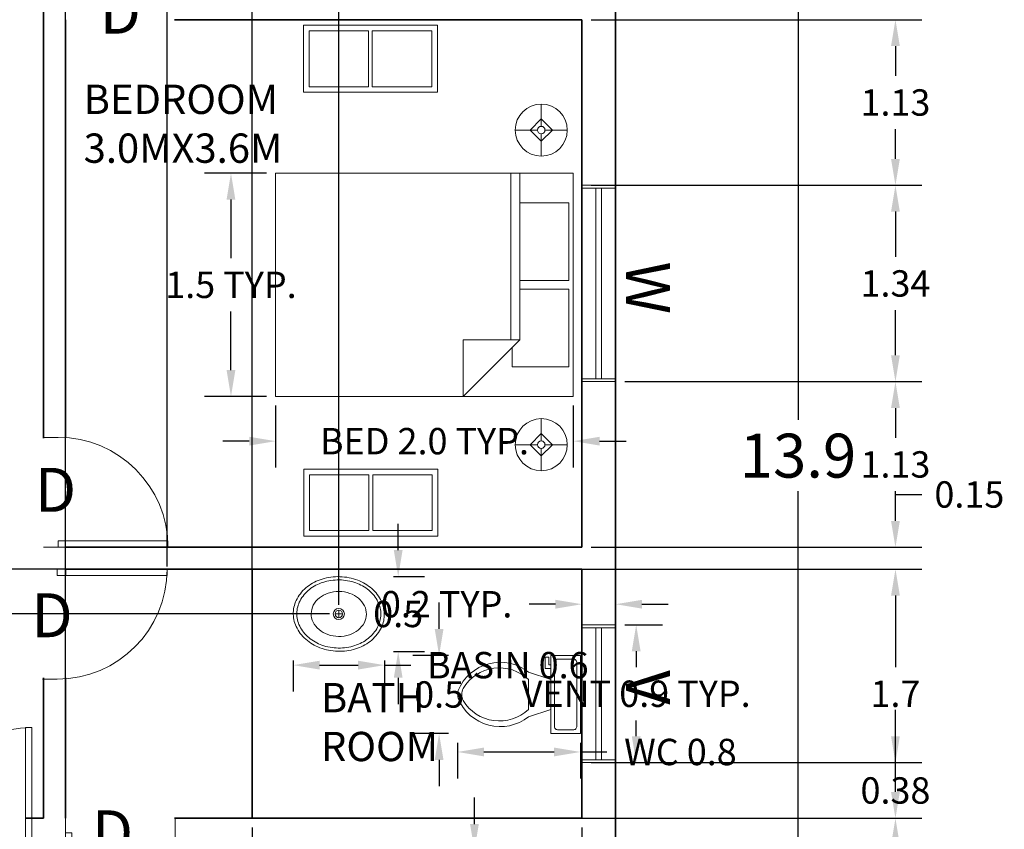
# Model space of a CAD drawing. Units: metres. Extents: x 40.9 to 56.1, y -1.4 to 24.2.
# Tile 5 of 7: x 48.4 to 55.2, y 13.1 to 18.6. Entities that reach past the tile are written whole.
import ezdxf

# ---------------------------------------------------------------- set-up
doc = ezdxf.new("R2010")
doc.units = ezdxf.units.M
doc.header["$MEASUREMENT"] = 0
for name, color, linetype, lineweight in [('A-ANNO-DIMS', 2, 'Continuous', 18), ('A-ANNO-TEXT', 7, 'Continuous', 18), ('A-AREA-IDEN', 7, 'Continuous', 18), ('A-DOOR', 3, 'Continuous', 18), ('A-FLOR-CASE', 9, 'Continuous', 18), ('A-FLOR-FIXT', 9, 'Continuous', 18), ('A-FURN', 8, 'Continuous', 18), ('A-GLAZ', 4, 'Continuous', 18), ('A-WALL', 7, 'Continuous', 35)]:
    doc.layers.add(name, color=color, linetype=linetype, lineweight=lineweight)
doc.styles.get("Standard").update_dxf_attribs({"font": 'arial.ttf'})
doc.dimstyles.get("Standard").update_dxf_attribs({"dimtxt": 0.18, "dimasz": 0.18, "dimexe": 0.18, "dimexo": 0.0625, "dimgap": 0.09, "dimtad": 0, "dimtih": 1, "dimtoh": 1, "dimdec": 1, "dimzin": 0, "dimdsep": 46, "dimtxsty": 'Standard', "dimcen": 0.09, "dimadec": 0, "dimazin": 0, "dimtfac": 1, "dimtdec": 1, "dimtofl": 0, "dimtmove": 0, "dimatfit": 3, "dimfxl": 1, "dimtolj": 1, "dimtzin": 0, "dimarcsym": 0})

# ---------------------------------------------------------------- blocks, each defined once
blk = doc.blocks.new('*U3')
for p, q in [((-750, 0), (-750, -100)), ((0, 0), (0, -100))]:
    blk.add_line(p, q)
blk.add_lwpolyline([(0, 0), (0, 750), (-43.75, 750), (-43.75, 0)], close=True)
blk.add_arc((0, 0), 750, 90, 180)
blk = doc.blocks.new('*U4')
for p, q in [((0, 0), (0, 100)), ((750, 0), (750, 100))]:
    blk.add_line(p, q)
blk.add_lwpolyline([(0, 0), (0, -750), (43.75, -750), (43.75, 0)], close=True)
blk.add_arc((0, 0), 750, 270, 0)
blk = doc.blocks.new('*U5')
for p, q in [((-750, 0), (-750, 100)), ((0, 0), (0, 100))]:
    blk.add_line(p, q)
blk.add_lwpolyline([(0, 0), (0, -750), (-43.75, -750), (-43.75, 0)], close=True)
blk.add_arc((0, 0), 750, 180, 270)
blk = doc.blocks.new('*U6')
for p, q in [((0, 0), (0, 100)), ((750, 0), (750, 100))]:
    blk.add_line(p, q)
blk.add_lwpolyline([(0, 0), (0, -750), (43.75, -750), (43.75, 0)], close=True)
blk.add_arc((0, 0), 750, 270, 0)
blk = doc.blocks.new('Bed - Queen')
for p, q in [((0, -80.00003), (0, 0)), ((0, 0), (59.99999, 0)), ((59.99999, 0), (59.99999, -80.00003)), ((7.99999, -1.2), (28.79998, -1.2)), ((7.99999, -14.4), (7.99999, -1.2)), ((28.79998, -1.2), (28.79998, -14.4)), ((31.19999, -1.2), (51.99999, -1.2)), ((31.19999, -14.4), (31.19999, -1.2)), ((51.99999, -1.2), (51.99999, -16.4)), ((0, -14.4), (44.8, -14.4)), ((59.99999, -29.6), (44.8, -14.4)), ((44.8, -14.4), (44.8, -29.6)), ((44.8, -16.8), (0, -16.8)), ((51.99999, -16.4), (46.79936, -16.4)), ((44.8, -29.6), (59.99999, -29.6)), ((59.99999, -80.00003), (0, -80.00003))]:
    blk.add_line(p, q)
blk = doc.blocks.new('Lamp - Table')
for p, q in [((0, 7), (0, 1)), ((0, 3), (-3, 0)), ((3, 0), (0, 3)), ((-1, 0), (-7, 0)), ((-3, 0), (0, -3)), ((0, -3), (3, 0)), ((1, 0), (7, 0)), ((0, -1), (0, -7))]:
    blk.add_line(p, q)
for radius in [7, 1]:
    blk.add_circle((0, 0), radius)
blk = doc.blocks.new('Toilet - top')
for p, q in [((9.5, -6), (9.5, -2)), ((-10, -8.5), (-8, -8.5)), ((-10, -9.5), (-10, -8.5)), ((-7, -9.5), (-10, -9.5)), ((-8, -8.5), (-8, -8)), ((-7, -8), (-7, -9.5)), ((-4, -8), (-6, -14)), ((4, -8), (6, -14)), ((4, -14), (-4, -14))]:
    blk.add_line(p, q)
blk.add_lwpolyline([(10.5, -8), (10.5, 0), (-10.5, 0), (-10.5, -8)], close=True)
for points in [[(-9.5, -2), (-9.5, -6)], [(8.5, -1), (-8.5, -1)], [(-8.5, -7), (8.5, -7)]]:
    blk.add_lwpolyline(points)
for centre, radius, start, end in [((-8.62, -1.88), 0.884, 81.8699, 188.1301), ((8.62, -1.88), 0.884, 351.8699, 98.1301), ((-8.62, -6.12), 0.884, 171.8699, 278.1301), ((8.62, -6.12), 0.884, 261.8699, 8.1301), ((3.52, -21.58), 12.17, 141.4691, 247.9714), ((4.2, -21.82), 11.33, 136.3677, 238.9468), ((-3.52, -21.58), 12.17, 292.0284, 38.5307), ((-4.2, -21.82), 11.33, 301.053, 43.6321), ((0, -27.88), 4, 245.7318, 294.2682), ((0, -29), 4, 254.8605, 285.1395)]:
    blk.add_arc(centre, radius, start, end)
blk = doc.blocks.new('Sink - Oval top')
for p, q in [((-1, 0), (1, 0)), ((0, 1), (0, -1))]:
    blk.add_line(p, q)
for points in [[(-12.23, 0.39, 0.117634), (-11.46, -3.36, 0.104469), (-8.88, -6.8, 0.090016), (-5.08, -9.07, 0.08192), (-0.32, -10.02, 0.08192), (4.49, -9.38, 0.090016), (8.42, -7.36, 0.104469), (11.22, -4.09, 0.117634), (12.23, -0.39, 0.117634), (11.46, 3.36, 0.104469), (8.88, 6.8, 0.090016), (5.08, 9.07, 0.08192), (0.32, 10.02, 0.08192), (-4.49, 9.38, 0.090016), (-8.42, 7.36, 0.104469), (-11.22, 4.09, 0.117634)], [(-11.29, 0.16, 0.118622), (-10.52, -3.25, 0.104678), (-8.07, -6.36, 0.089562), (-4.54, -8.37, 0.081185), (-0.13, -9.15, 0.081185), (4.3, -8.49, 0.089562), (7.89, -6.58, 0.104678), (10.42, -3.55, 0.118622), (11.29, -0.16, 0.118622), (10.52, 3.25, 0.104678), (8.07, 6.36, 0.089562), (4.54, 8.37, 0.081185), (0.13, 9.15, 0.081185), (-4.3, 8.49, 0.089562), (-7.89, 6.58, 0.104678), (-10.42, 3.55, 0.118622)], [(-7.42, 0.08, 0.118283), (-6.91, -2.17, 0.104607), (-5.29, -4.21, 0.089718), (-2.97, -5.53, 0.081436), (-0.07, -6.04, 0.081436), (2.84, -5.59, 0.089718), (5.2, -4.33, 0.104607), (6.86, -2.32, 0.118283), (7.42, -0.08, 0.118283), (6.91, 2.17, 0.104607), (5.29, 4.21, 0.089718), (2.97, 5.53, 0.081436), (0.07, 6.04, 0.081436), (-2.84, 5.59, 0.089718), (-5.2, 4.33, 0.104607), (-6.86, 2.32, 0.118283)]]:
    blk.add_lwpolyline(points, format="xyb", close=True)
for radius in [1.5, 1]:
    blk.add_circle((0, 0), radius)
blk = doc.blocks.new('Wall Cabinet - 18 x 36 in front')
for p, q in [((17.5, -1.5), (17.5, -16.5)), ((18.5, -16.5), (18.5, -1.5))]:
    blk.add_line(p, q)
blk.add_lwpolyline([(0, -18), (0, 0), (36, 0), (36, -18)], close=True)
for points in [[(17.5, -16.5), (1.5, -16.5), (1.5, -1.5), (17.5, -1.5)], [(18.5, -1.5), (34.5, -1.5), (34.5, -16.5), (18.5, -16.5)]]:
    blk.add_lwpolyline(points)
blk = doc.blocks.new('*D46')
at = {"layer": 'A-ANNO-DIMS', "color": 0, "lineweight": -2, "transparency": 16777216}
for p, q in [((52.5777, 22.5873), (53.9408, 22.5873)), ((53.7608, 22.2873), (53.7608, 15.8755)), ((53.7608, 8.9773), (53.7608, 15.389)), ((52.5777, 8.6773), (53.9408, 8.6773))]:
    blk.add_line(p, q, dxfattribs=at)
at = {"layer": 'A-ANNO-DIMS', "color": 0, "transparency": 16777216}
for points in [[(53.7108, 22.2873), (53.8108, 22.2873), (53.7608, 22.5873)], [(53.7108, 8.9773), (53.8108, 8.9773), (53.7608, 8.6773)]]:
    blk.add_solid(points, dxfattribs=at)
at = {"layer": 'Defpoints', "color": 0, "transparency": 16777216}
for p in [(52.5152, 22.5873), (52.5152, 8.6773), (53.7608, 8.6773)]:
    blk.add_point(p, dxfattribs=at)
at = {"layer": 'A-ANNO-DIMS', "color": 0, "transparency": 16777216, "insert": (53.7608, 15.6323), "char_height": 0.3, "attachment_point": 5}
blk.add_mtext('\\A1;13.9', dxfattribs=at)
blk = doc.blocks.new('VENT-900-PLAN')
for p, q in [((0.0002, 0.0003), (0.0002, 0.2303)), ((0.0202, 0.0003), (0.0202, 0.2303)), ((0.9202, 0.0003), (0.9202, 0.2303)), ((0.9402, 0.0003), (0.9402, 0.2303)), ((0.0202, 0.1353), (0.9202, 0.1353)), ((0.0202, 0.0953), (0.9202, 0.0953))]:
    blk.add_line(p, q)
blk = doc.blocks.new('*D75')
at = {"layer": 'A-ANNO-DIMS', "color": 0, "lineweight": -2, "transparency": 16777216}
for p, q in [((52.5777, 14.4773), (52.8362, 14.4773)), ((52.6562, 14.2973), (52.6562, 14.1892)), ((52.6562, 13.7173), (52.6562, 13.8254)), ((52.5777, 13.5373), (52.8362, 13.5373))]:
    blk.add_line(p, q, dxfattribs=at)
at = {"layer": 'A-ANNO-DIMS', "color": 0, "transparency": 16777216}
for points in [[(52.6262, 14.2973), (52.6862, 14.2973), (52.6562, 14.4773)], [(52.6262, 13.7173), (52.6862, 13.7173), (52.6562, 13.5373)]]:
    blk.add_solid(points, dxfattribs=at)
at = {"layer": 'Defpoints', "color": 0, "transparency": 16777216}
for p in [(52.5152, 14.4773), (52.6562, 14.4773), (52.5152, 13.5373)]:
    blk.add_point(p, dxfattribs=at)
at = {"layer": 'A-ANNO-DIMS', "color": 0, "transparency": 16777216, "insert": (52.6562, 14.0073), "char_height": 0.18, "attachment_point": 5}
blk.add_mtext('\\A1;VENT 0.9 TYP.', dxfattribs=at)
blk = doc.blocks.new('*D76')
at = {"layer": 'A-ANNO-DIMS', "color": 0, "lineweight": -2, "transparency": 16777216}
for p, q in [((52.2852, 14.5398), (52.2852, 14.7983)), ((52.5152, 14.5398), (52.5152, 14.7983)), ((52.1052, 14.6183), (51.9252, 14.6183)), ((52.6952, 14.6183), (52.8752, 14.6183))]:
    blk.add_line(p, q, dxfattribs=at)
at = {"layer": 'A-ANNO-DIMS', "color": 0, "transparency": 16777216}
for points in [[(52.1052, 14.6483), (52.1052, 14.5883), (52.2852, 14.6183)], [(52.6952, 14.6483), (52.6952, 14.5883), (52.5152, 14.6183)]]:
    blk.add_solid(points, dxfattribs=at)
at = {"layer": 'Defpoints', "color": 0, "transparency": 16777216}
for p in [(52.2852, 14.6183), (52.2852, 14.4773), (52.5152, 14.4773)]:
    blk.add_point(p, dxfattribs=at)
at = {"layer": 'A-ANNO-DIMS', "color": 0, "transparency": 16777216, "insert": (51.3622, 14.6183), "char_height": 0.18, "attachment_point": 5}
blk.add_mtext('\\A1;0.2 TYP.', dxfattribs=at)
blk = doc.blocks.new('*D79')
at = {"layer": 'A-ANNO-DIMS', "color": 0, "lineweight": -2, "transparency": 16777216}
for p, q in [((50.1947, 15.9733), (50.1947, 15.551)), ((52.2267, 15.9733), (52.2267, 15.551)), ((50.0147, 15.731), (49.8347, 15.731)), ((52.4067, 15.731), (52.5867, 15.731))]:
    blk.add_line(p, q, dxfattribs=at)
at = {"layer": 'A-ANNO-DIMS', "color": 0, "transparency": 16777216}
for points in [[(50.0147, 15.761), (50.0147, 15.701), (50.1947, 15.731)], [(52.4067, 15.761), (52.4067, 15.701), (52.2267, 15.731)]]:
    blk.add_solid(points, dxfattribs=at)
at = {"layer": 'Defpoints', "color": 0, "transparency": 16777216}
for p in [(50.1947, 16.0358), (52.2267, 16.0358), (52.2267, 15.731)]:
    blk.add_point(p, dxfattribs=at)
at = {"layer": 'A-ANNO-DIMS', "color": 0, "transparency": 16777216, "insert": (51.2107, 15.731), "char_height": 0.18, "attachment_point": 5}
blk.add_mtext('\\A1;BED 2.0 TYP.', dxfattribs=at)
blk = doc.blocks.new('*D80')
at = {"layer": 'A-ANNO-DIMS', "color": 0, "lineweight": -2, "transparency": 16777216}
for p, q in [((50.1322, 17.5598), (49.7099, 17.5598)), ((49.8899, 17.3798), (49.8899, 16.9798)), ((49.8899, 16.2158), (49.8899, 16.6159)), ((50.1322, 16.0358), (49.7099, 16.0358))]:
    blk.add_line(p, q, dxfattribs=at)
at = {"layer": 'A-ANNO-DIMS', "color": 0, "transparency": 16777216}
for points in [[(49.8599, 17.3798), (49.9199, 17.3798), (49.8899, 17.5598)], [(49.8599, 16.2158), (49.9199, 16.2158), (49.8899, 16.0358)]]:
    blk.add_solid(points, dxfattribs=at)
at = {"layer": 'Defpoints', "color": 0, "transparency": 16777216}
for p in [(50.1947, 17.5598), (49.8899, 16.0358), (50.1947, 16.0358)]:
    blk.add_point(p, dxfattribs=at)
at = {"layer": 'A-ANNO-DIMS', "color": 0, "transparency": 16777216, "insert": (49.8899, 16.7978), "char_height": 0.18, "attachment_point": 5}
blk.add_mtext('\\A1;1.5 TYP.', dxfattribs=at)
blk = doc.blocks.new('*D86')
at = {"layer": 'A-ANNO-DIMS', "color": 0, "lineweight": -2, "transparency": 16777216}
for p, q in [((51.5519, 13.1183), (51.5519, 13.2983)), ((51.4772, 12.9383), (51.7319, 12.9383)), ((51.4772, 12.4811), (51.7319, 12.4811)), ((51.5519, 12.3011), (51.5519, 12.1211))]:
    blk.add_line(p, q, dxfattribs=at)
at = {"layer": 'A-ANNO-DIMS', "color": 0, "transparency": 16777216}
for points in [[(51.5219, 13.1183), (51.5819, 13.1183), (51.5519, 12.9383)], [(51.5219, 12.3011), (51.5819, 12.3011), (51.5519, 12.4811)]]:
    blk.add_solid(points, dxfattribs=at)
at = {"layer": 'Defpoints', "color": 0, "transparency": 16777216}
for p in [(51.4147, 12.9383), (51.5519, 12.9383), (51.4147, 12.4811)]:
    blk.add_point(p, dxfattribs=at)
at = {"layer": 'A-ANNO-DIMS', "color": 0, "transparency": 16777216, "insert": (51.5519, 12.7097), "char_height": 0.18, "attachment_point": 5}
blk.add_mtext('\\A1;0.5 TYP.', dxfattribs=at)
blk = doc.blocks.new('*D91')
at = {"layer": 'A-ANNO-DIMS', "color": 0, "lineweight": -2, "transparency": 16777216}
for p, q in [((51.4367, 13.6733), (51.4367, 13.4299)), ((52.2761, 13.6733), (52.2761, 13.4299)), ((51.6167, 13.6099), (52.0961, 13.6099)), ((52.2761, 13.6099), (52.4561, 13.6099))]:
    blk.add_line(p, q, dxfattribs=at)
at = {"layer": 'A-ANNO-DIMS', "color": 0, "transparency": 16777216}
for points in [[(51.6167, 13.6399), (51.6167, 13.5799), (51.4367, 13.6099)], [(52.0961, 13.6399), (52.0961, 13.5799), (52.2761, 13.6099)]]:
    blk.add_solid(points, dxfattribs=at)
at = {"layer": 'Defpoints', "color": 0, "transparency": 16777216}
for p in [(51.4367, 13.7358), (52.2761, 13.7358), (52.2761, 13.6099)]:
    blk.add_point(p, dxfattribs=at)
at = {"layer": 'A-ANNO-DIMS', "color": 0, "transparency": 16777216, "insert": (52.9582, 13.6099), "char_height": 0.18, "attachment_point": 5}
blk.add_mtext('\\A1;WC 0.8', dxfattribs=at)
blk = doc.blocks.new('*D92')
at = {"layer": 'A-ANNO-DIMS', "color": 0, "lineweight": -2, "transparency": 16777216}
for p, q in [((51.3108, 14.4492), (51.3108, 14.6292)), ((51.3742, 14.2692), (51.1308, 14.2692)), ((51.3742, 13.7358), (51.1308, 13.7358)), ((51.3108, 13.5558), (51.3108, 13.3758))]:
    blk.add_line(p, q, dxfattribs=at)
at = {"layer": 'A-ANNO-DIMS', "color": 0, "transparency": 16777216}
for points in [[(51.2808, 14.4492), (51.3408, 14.4492), (51.3108, 14.2692)], [(51.2808, 13.5558), (51.3408, 13.5558), (51.3108, 13.7358)]]:
    blk.add_solid(points, dxfattribs=at)
at = {"layer": 'Defpoints', "color": 0, "transparency": 16777216}
for p in [(51.4367, 14.2692), (51.3108, 13.7358), (51.4367, 13.7358)]:
    blk.add_point(p, dxfattribs=at)
at = {"layer": 'A-ANNO-DIMS', "color": 0, "transparency": 16777216, "insert": (51.3108, 14.0025), "char_height": 0.18, "attachment_point": 5}
blk.add_mtext('\\A1;0.5', dxfattribs=at)
blk = doc.blocks.new('*D95')
at = {"layer": 'A-ANNO-DIMS', "color": 0, "lineweight": -2, "transparency": 16777216}
for p, q in [((50.3144, 14.2336), (50.3144, 14.0225)), ((50.4944, 14.2025), (50.7579, 14.2025)), ((50.9379, 14.2336), (50.9379, 14.0225)), ((50.9379, 14.2025), (51.1179, 14.2025))]:
    blk.add_line(p, q, dxfattribs=at)
at = {"layer": 'A-ANNO-DIMS', "color": 0, "transparency": 16777216}
for points in [[(50.4944, 14.2325), (50.4944, 14.1725), (50.3144, 14.2025)], [(50.7579, 14.2325), (50.7579, 14.1725), (50.9379, 14.2025)]]:
    blk.add_solid(points, dxfattribs=at)
at = {"layer": 'Defpoints', "color": 0, "transparency": 16777216}
for p in [(50.3144, 14.2961), (50.9379, 14.2961), (50.9379, 14.2025)]:
    blk.add_point(p, dxfattribs=at)
at = {"layer": 'A-ANNO-DIMS', "color": 0, "transparency": 16777216, "insert": (51.78, 14.2025), "char_height": 0.18, "attachment_point": 5}
blk.add_mtext('\\A1;BASIN 0.6', dxfattribs=at)
blk = doc.blocks.new('*D96')
at = {"layer": 'A-ANNO-DIMS', "color": 0, "lineweight": -2, "transparency": 16777216}
for p, q in [((51.0315, 14.9875), (51.0315, 15.1675)), ((51.0004, 14.8075), (51.2115, 14.8075)), ((51.0004, 14.2961), (51.2115, 14.2961)), ((51.0315, 14.1161), (51.0315, 13.9361))]:
    blk.add_line(p, q, dxfattribs=at)
at = {"layer": 'A-ANNO-DIMS', "color": 0, "transparency": 16777216}
for points in [[(51.0015, 14.9875), (51.0615, 14.9875), (51.0315, 14.8075)], [(51.0015, 14.1161), (51.0615, 14.1161), (51.0315, 14.2961)]]:
    blk.add_solid(points, dxfattribs=at)
at = {"layer": 'Defpoints', "color": 0, "transparency": 16777216}
for p in [(50.9379, 14.8075), (51.0315, 14.8075), (50.9379, 14.2961)]:
    blk.add_point(p, dxfattribs=at)
at = {"layer": 'A-ANNO-DIMS', "color": 0, "transparency": 16777216, "insert": (51.0315, 14.5518), "char_height": 0.18, "attachment_point": 5}
blk.add_mtext('\\A1;0.5', dxfattribs=at)
blk = doc.blocks.new('*D134')
at = {"layer": 'A-ANNO-DIMS', "color": 0, "lineweight": -2, "transparency": 16777216}
for p, q in [((50.034, 13.0948), (50.034, 6.6791)), ((52.2852, 13.0948), (52.2852, 6.6791)), ((50.214, 6.8591), (50.8336, 6.8591)), ((52.1052, 6.8591), (51.4856, 6.8591))]:
    blk.add_line(p, q, dxfattribs=at)
at = {"layer": 'A-ANNO-DIMS', "color": 0, "transparency": 16777216}
for points in [[(50.214, 6.8891), (50.214, 6.8291), (50.034, 6.8591)], [(52.1052, 6.8891), (52.1052, 6.8291), (52.2852, 6.8591)]]:
    blk.add_solid(points, dxfattribs=at)
at = {"layer": 'Defpoints', "color": 0, "transparency": 16777216}
for p in [(50.034, 13.1573), (52.2852, 13.1573), (52.2852, 6.8591)]:
    blk.add_point(p, dxfattribs=at)
at = {"layer": 'A-ANNO-DIMS', "color": 0, "transparency": 16777216, "insert": (51.1596, 6.8591), "char_height": 0.18, "attachment_point": 5}
blk.add_mtext('\\A1;2.25', dxfattribs=at)
blk = doc.blocks.new('*D135')
at = {"layer": 'A-ANNO-DIMS', "color": 0, "lineweight": -2, "transparency": 16777216}
for p, q in [((50.0965, 14.8573), (54.6058, 14.8573)), ((54.4258, 14.6773), (54.4258, 14.1876)), ((54.4258, 13.3373), (54.4258, 13.8269)), ((50.0965, 13.1573), (54.6058, 13.1573))]:
    blk.add_line(p, q, dxfattribs=at)
at = {"layer": 'A-ANNO-DIMS', "color": 0, "transparency": 16777216}
for points in [[(54.3958, 14.6773), (54.4558, 14.6773), (54.4258, 14.8573)], [(54.3958, 13.3373), (54.4558, 13.3373), (54.4258, 13.1573)]]:
    blk.add_solid(points, dxfattribs=at)
at = {"layer": 'Defpoints', "color": 0, "transparency": 16777216}
for p in [(50.034, 14.8573), (54.4258, 14.8573), (50.034, 13.1573)]:
    blk.add_point(p, dxfattribs=at)
at = {"layer": 'A-ANNO-DIMS', "color": 0, "transparency": 16777216, "insert": (54.4258, 14.0073), "char_height": 0.18, "attachment_point": 5}
blk.add_mtext('\\A1;1.7', dxfattribs=at)
blk = doc.blocks.new('*D136')
at = {"layer": 'A-ANNO-DIMS', "color": 0, "lineweight": -2, "transparency": 16777216}
for p, q in [((48.7602, 14.8764), (48.7602, 24.2418)), ((49.4546, 14.8764), (49.4546, 24.2418)), ((48.5802, 24.0618), (48.4002, 24.0618)), ((49.6346, 24.0618), (49.8146, 24.0618))]:
    blk.add_line(p, q, dxfattribs=at)
at = {"layer": 'A-ANNO-DIMS', "color": 0, "transparency": 16777216}
for points in [[(48.5802, 24.0918), (48.5802, 24.0318), (48.7602, 24.0618)], [(49.6346, 24.0918), (49.6346, 24.0318), (49.4546, 24.0618)]]:
    blk.add_solid(points, dxfattribs=at)
at = {"layer": 'Defpoints', "color": 0, "transparency": 16777216}
for p in [(49.4546, 24.0618), (48.7602, 14.8139), (49.4546, 14.8139)]:
    blk.add_point(p, dxfattribs=at)
at = {"layer": 'A-ANNO-DIMS', "color": 0, "transparency": 16777216, "insert": (49.1074, 24.0618), "char_height": 0.18, "attachment_point": 5}
blk.add_mtext('\\A1;0.69', dxfattribs=at)
blk = doc.blocks.new('*D140')
at = {"layer": 'A-ANNO-DIMS', "color": 0, "lineweight": -2, "transparency": 16777216}
for p, q in [((52.5777, 16.1373), (54.6058, 16.1373)), ((54.4258, 15.9573), (54.4258, 15.7542)), ((54.4258, 15.1873), (54.4258, 15.3903)), ((52.3477, 15.0073), (54.6058, 15.0073))]:
    blk.add_line(p, q, dxfattribs=at)
at = {"layer": 'A-ANNO-DIMS', "color": 0, "transparency": 16777216}
for points in [[(54.3958, 15.9573), (54.4558, 15.9573), (54.4258, 16.1373)], [(54.3958, 15.1873), (54.4558, 15.1873), (54.4258, 15.0073)]]:
    blk.add_solid(points, dxfattribs=at)
at = {"layer": 'Defpoints', "color": 0, "transparency": 16777216}
for p in [(52.5152, 16.1373), (54.4258, 16.1373), (52.2852, 15.0073)]:
    blk.add_point(p, dxfattribs=at)
at = {"layer": 'A-ANNO-DIMS', "color": 0, "transparency": 16777216, "insert": (54.4258, 15.5723), "char_height": 0.18, "attachment_point": 5}
blk.add_mtext('\\A1;1.13', dxfattribs=at)
blk = doc.blocks.new('*D141')
at = {"layer": 'A-ANNO-DIMS', "color": 0, "lineweight": -2, "transparency": 16777216}
for p, q in [((52.5777, 17.4773), (54.6058, 17.4773)), ((54.4258, 17.2973), (54.4258, 16.9892)), ((54.4258, 16.3173), (54.4258, 16.6253)), ((52.5777, 16.1373), (54.6058, 16.1373))]:
    blk.add_line(p, q, dxfattribs=at)
at = {"layer": 'A-ANNO-DIMS', "color": 0, "transparency": 16777216}
for points in [[(54.3958, 17.2973), (54.4558, 17.2973), (54.4258, 17.4773)], [(54.3958, 16.3173), (54.4558, 16.3173), (54.4258, 16.1373)]]:
    blk.add_solid(points, dxfattribs=at)
at = {"layer": 'Defpoints', "color": 0, "transparency": 16777216}
for p in [(52.5152, 17.4773), (54.4258, 17.4773), (52.5152, 16.1373)]:
    blk.add_point(p, dxfattribs=at)
at = {"layer": 'A-ANNO-DIMS', "color": 0, "transparency": 16777216, "insert": (54.4258, 16.8073), "char_height": 0.18, "attachment_point": 5}
blk.add_mtext('\\A1;1.34', dxfattribs=at)
blk = doc.blocks.new('*D150')
at = {"layer": 'A-ANNO-DIMS', "color": 0, "lineweight": -2, "transparency": 16777216}
for p, q in [((50.034, 14.9198), (50.034, 24.2418)), ((50.6262, 14.6143), (50.6262, 24.2418)), ((50.214, 24.0618), (50.4462, 24.0618)), ((50.6262, 24.0618), (50.8062, 24.0618))]:
    blk.add_line(p, q, dxfattribs=at)
at = {"layer": 'A-ANNO-DIMS', "color": 0, "transparency": 16777216}
for points in [[(50.214, 24.0918), (50.214, 24.0318), (50.034, 24.0618)], [(50.4462, 24.0918), (50.4462, 24.0318), (50.6262, 24.0618)]]:
    blk.add_solid(points, dxfattribs=at)
at = {"layer": 'Defpoints', "color": 0, "transparency": 16777216}
for p in [(50.6262, 24.0618), (50.034, 14.8573), (50.6262, 14.5518)]:
    blk.add_point(p, dxfattribs=at)
at = {"layer": 'A-ANNO-DIMS', "color": 0, "transparency": 16777216, "insert": (51.1301, 24.0618), "char_height": 0.18, "attachment_point": 5}
blk.add_mtext('\\A1;0.59', dxfattribs=at)
blk = doc.blocks.new('*D151')
at = {"layer": 'A-ANNO-DIMS', "color": 0, "lineweight": -2, "transparency": 16777216}
for p, q in [((43.3221, 15.0373), (43.3221, 15.2173)), ((49.9715, 14.8573), (43.1421, 14.8573)), ((50.5637, 14.5518), (43.1421, 14.5518)), ((43.3221, 14.3718), (43.3221, 14.1918)), ((43.3221, 14.1918), (43.1421, 14.1918))]:
    blk.add_line(p, q, dxfattribs=at)
at = {"layer": 'A-ANNO-DIMS', "color": 0, "transparency": 16777216}
for points in [[(43.2921, 15.0373), (43.3521, 15.0373), (43.3221, 14.8573)], [(43.2921, 14.3718), (43.3521, 14.3718), (43.3221, 14.5518)]]:
    blk.add_solid(points, dxfattribs=at)
at = {"layer": 'Defpoints', "color": 0, "transparency": 16777216}
for p in [(50.034, 14.8573), (43.3221, 14.5518), (50.6262, 14.5518)]:
    blk.add_point(p, dxfattribs=at)
at = {"layer": 'A-ANNO-DIMS', "color": 0, "transparency": 16777216, "insert": (42.8357, 14.1918), "char_height": 0.18, "attachment_point": 5}
blk.add_mtext('\\A1;0.31', dxfattribs=at)
blk = doc.blocks.new('*D152')
at = {"layer": 'A-ANNO-DIMS', "color": 0, "lineweight": -2, "transparency": 16777216}
for p, q in [((54.42584, 13.717253), (54.42584, 13.897253)), ((52.347703, 13.537253), (54.60584, 13.537253)), ((52.347703, 13.157253), (54.60584, 13.157253)), ((54.42584, 12.977253), (54.42584, 12.797253))]:
    blk.add_line(p, q, dxfattribs=at)
at = {"layer": 'A-ANNO-DIMS', "color": 0, "transparency": 16777216}
for points in [[(54.39584, 13.717253), (54.45584, 13.717253), (54.42584, 13.537253)], [(54.39584, 12.977253), (54.45584, 12.977253), (54.42584, 13.157253)]]:
    blk.add_solid(points, dxfattribs=at)
at = {"layer": 'Defpoints', "color": 0, "transparency": 16777216}
for p in [(52.285203, 13.537253), (54.42584, 13.537253), (52.285203, 13.157253)]:
    blk.add_point(p, dxfattribs=at)
at = {"layer": 'A-ANNO-DIMS', "color": 0, "transparency": 16777216, "insert": (54.42584, 13.347253), "char_height": 0.18, "attachment_point": 5}
blk.add_mtext('\\A1;0.38', dxfattribs=at)
blk = doc.blocks.new('*D153')
at = {"layer": 'A-ANNO-DIMS', "color": 0, "lineweight": -2, "transparency": 16777216}
for p, q in [((54.4258, 15.1873), (54.4258, 15.3673)), ((54.4258, 15.3673), (54.6058, 15.3673)), ((52.3477, 15.0073), (54.6058, 15.0073)), ((52.3477, 14.8573), (54.6058, 14.8573)), ((54.4258, 14.6773), (54.4258, 14.4973))]:
    blk.add_line(p, q, dxfattribs=at)
at = {"layer": 'A-ANNO-DIMS', "color": 0, "transparency": 16777216}
for points in [[(54.3958, 15.1873), (54.4558, 15.1873), (54.4258, 15.0073)], [(54.3958, 14.6773), (54.4558, 14.6773), (54.4258, 14.8573)]]:
    blk.add_solid(points, dxfattribs=at)
at = {"layer": 'Defpoints', "color": 0, "transparency": 16777216}
for p in [(52.2852, 15.0073), (54.4258, 15.0073), (52.2852, 14.8573)]:
    blk.add_point(p, dxfattribs=at)
at = {"layer": 'A-ANNO-DIMS', "color": 0, "transparency": 16777216, "insert": (54.9303, 15.3673), "char_height": 0.18, "attachment_point": 5}
blk.add_mtext('\\A1;0.15', dxfattribs=at)
blk = doc.blocks.new('*D154')
at = {"layer": 'A-ANNO-DIMS', "color": 0, "lineweight": -2, "transparency": 16777216}
for p, q in [((48.7602, 13.2198), (48.7602, 24.2418)), ((50.034, 13.2198), (50.034, 24.2418)), ((48.9402, 24.0618), (49.0818, 24.0618)), ((49.854, 24.0618), (49.7124, 24.0618))]:
    blk.add_line(p, q, dxfattribs=at)
at = {"layer": 'A-ANNO-DIMS', "color": 0, "transparency": 16777216}
for points in [[(48.9402, 24.0918), (48.9402, 24.0318), (48.7602, 24.0618)], [(49.854, 24.0918), (49.854, 24.0318), (50.034, 24.0618)]]:
    blk.add_solid(points, dxfattribs=at)
at = {"layer": 'Defpoints', "color": 0, "transparency": 16777216}
for p in [(50.034, 24.0618), (48.7602, 13.1573), (50.034, 13.1573)]:
    blk.add_point(p, dxfattribs=at)
at = {"layer": 'A-ANNO-DIMS', "color": 0, "transparency": 16777216, "insert": (49.3971, 24.0618), "char_height": 0.18, "attachment_point": 5}
blk.add_mtext('\\A1;1.27', dxfattribs=at)
blk = doc.blocks.new('*D159')
at = {"layer": 'A-ANNO-DIMS', "color": 0, "lineweight": -2, "transparency": 16777216}
for p, q in [((52.3477, 18.6073), (54.6058, 18.6073)), ((54.4258, 18.4273), (54.4258, 18.2242)), ((54.4258, 17.6573), (54.4258, 17.8603)), ((52.3477, 17.4773), (54.6058, 17.4773))]:
    blk.add_line(p, q, dxfattribs=at)
at = {"layer": 'A-ANNO-DIMS', "color": 0, "transparency": 16777216}
for points in [[(54.3958, 18.4273), (54.4558, 18.4273), (54.4258, 18.6073)], [(54.3958, 17.6573), (54.4558, 17.6573), (54.4258, 17.4773)]]:
    blk.add_solid(points, dxfattribs=at)
at = {"layer": 'Defpoints', "color": 0, "transparency": 16777216}
for p in [(52.2852, 18.6073), (54.4258, 18.6073), (52.2852, 17.4773)]:
    blk.add_point(p, dxfattribs=at)
at = {"layer": 'A-ANNO-DIMS', "color": 0, "transparency": 16777216, "insert": (54.4258, 18.0423), "char_height": 0.18, "attachment_point": 5}
blk.add_mtext('\\A1;1.13', dxfattribs=at)

msp = doc.modelspace()

# ---------------------------------------------------------------- linework, layer by layer
at = {"layer": 'A-GLAZ'}
for p, q in [((52.2852, 17.4773), (52.5152, 17.4773)), ((52.2852, 17.4573), (52.5152, 17.4573)), ((52.3802, 17.4573), (52.3802, 16.1573)), ((52.4202, 17.4573), (52.4202, 16.1573)), ((52.2852, 16.1573), (52.5152, 16.1573)), ((52.2852, 16.1373), (52.5152, 16.1373))]:
    msp.add_line(p, q, dxfattribs=at)
at = {"layer": 'A-WALL'}
for p, q in [((48.6102, 19.7073), (48.6102, 15.7504)), ((52.5152, 18.7573), (52.5152, 13.1573)), ((48.7602, 18.6073), (48.7602, 15.7554)), ((52.2852, 18.6073), (49.5035, 18.6073)), ((52.2852, 18.6073), (52.2852, 15.0073)), ((52.2852, 15.0073), (48.7602, 15.0073)), ((52.2852, 14.8573), (48.7602, 14.8573)), ((48.7602, 14.8573), (48.7602, 14.8139)), ((50.034, 14.8573), (50.034, 13.1573)), ((52.2852, 14.8573), (52.2852, 13.1573)), ((48.6102, 14.1157), (48.6102, 13.1573)), ((48.7602, 14.1157), (48.7602, 13.1573)), ((48.4865, 13.1573), (48.6102, 13.1573)), ((49.5035, 13.1573), (52.2852, 13.1573)), ((52.5152, 8.6773), (52.5152, 13.1573))]:
    msp.add_line(p, q, dxfattribs=at)

# ---------------------------------------------------------------- block references
at = {"layer": 'A-DOOR', "xscale": 0.001, "yscale": 0.001, "zscale": 0.001, "rotation": 90}
for name, p in [('*U6', (48.7102, 15.0071)), ('*U5', (48.7046, 14.8577))]:
    msp.add_blockref(name, p, dxfattribs=at)
at = {"layer": 'A-DOOR', "xscale": 0.001, "yscale": 0.001, "zscale": 0.001}
for name, p in [('*U3', (48.5302, 13.0273)), ('*U4', (48.7602, 13.0573))]:
    msp.add_blockref(name, p, dxfattribs=at)
at = {"layer": 'A-FLOR-CASE', "xscale": 0.0254, "yscale": 0.0254, "zscale": 0.0254}
for p in [(50.3846, 18.569), (50.3876, 15.5398)]:
    msp.add_blockref('Wall Cabinet - 18 x 36 in front', p, dxfattribs=at)
at = {"layer": 'A-FLOR-FIXT', "xscale": 0.0254, "yscale": 0.0254, "zscale": 0.0254}
msp.add_blockref('Sink - Oval top', (50.6262, 14.5518), dxfattribs=at)
at = {"layer": 'A-FLOR-FIXT', "xscale": 0.0254, "yscale": 0.0254, "zscale": 0.0254, "rotation": 270}
msp.add_blockref('Toilet - top', (52.2761, 14.0025), dxfattribs=at)
at = {"layer": 'A-FURN', "xscale": 0.0254, "yscale": 0.0254, "zscale": 0.0254}
for p in [(52.0082, 17.8539), (52.0082, 15.7069)]:
    msp.add_blockref('Lamp - Table', p, dxfattribs=at)
at = {"layer": 'A-FURN', "xscale": 0.0254, "yscale": 0.0254, "zscale": 0.0254, "rotation": 270}
msp.add_blockref('Bed - Queen', (52.2267, 17.5598), dxfattribs=at)
at = {"layer": 'A-GLAZ', "rotation": 90.0000000000022}
msp.add_blockref('VENT-900-PLAN', (52.5155, 13.5371), dxfattribs=at)

# ---------------------------------------------------------------- texts
at = {"layer": 'A-ANNO-TEXT'}
for p in [(48.994, 18.5117), (48.5518, 15.2488), (48.528, 14.3929), (48.9405, 12.9118)]:
    msp.add_text('D ', height=0.3, dxfattribs=at).set_placement(p)
for s, p in [('W', (52.5874, 16.9571)), ('V', (52.5874, 14.1683))]:
    msp.add_text(s, height=0.3, rotation=270, dxfattribs=at).set_placement(p)
at = {"layer": 'A-AREA-IDEN', "char_height": 0.2, "attachment_point": 1}
for s, insert in [('BEDROOM\\P3.0MX3.6M', (48.8846, 18.164)), ('BATH\\PROOM', (50.5047, 14.0807))]:
    msp.add_mtext_dynamic_manual_height_columns(s, width=2.030673, gutter_width=1, heights=[0], dxfattribs=dict(at, insert=insert))

# ---------------------------------------------------------------- dimensions: what is measured, and where the dimension line sits
at = {"layer": 'A-ANNO-DIMS'}
for base, p1, p2, picture, middle in [((49.4546, 24.0618), (48.7602, 14.8139), (49.4546, 14.8139), '*D136', (49.1074, 24.0618)), ((50.034, 24.0618), (48.7602, 13.1573), (50.034, 13.1573), '*D154', (49.3971, 24.0618)), ((50.6262, 24.0618), (50.034, 14.8573), (50.6262, 14.5518), '*D150', (51.1301, 24.0618)), ((52.2852, 6.8591), (50.034, 13.1573), (52.2852, 13.1573), '*D134', (51.1596, 6.8591))]:
    dim = msp.add_linear_dim(base=base, p1=p1, p2=p2, dimstyle='Standard', override={"dimdec": 2, "dimlfac": 1, "dimrnd": 0, "dimzin": 0, "dimdsep": 46, "dimlunit": 2}, dxfattribs=at)
    dim.commit()
    dim.dimension.update_dxf_attribs({"geometry": picture, "text_midpoint": middle})
for base, p1, p2, angle, override, picture, middle in [((53.7608, 8.6773), (52.5152, 22.5873), (52.5152, 8.6773), 90, {"dimtxt": 0.3, "dimasz": 0.3, "dimclrd": 0, "dimclre": 0, "dimclrt": 0}, '*D46', (53.7608, 15.6323)), ((54.4258, 18.6073), (52.2852, 17.4773), (52.2852, 18.6073), 90, {"dimdec": 2, "dimlfac": 1, "dimrnd": 0, "dimzin": 0, "dimdsep": 46, "dimlunit": 2}, '*D159', (54.4258, 18.0423)), ((54.4258, 17.4773), (52.5152, 16.1373), (52.5152, 17.4773), 90, {"dimdec": 2, "dimlfac": 1, "dimrnd": 0, "dimzin": 0, "dimdsep": 46, "dimlunit": 2}, '*D141', (54.4258, 16.8073)), ((54.4258, 16.1373), (52.2852, 15.0073), (52.5152, 16.1373), 90, {"dimdec": 2, "dimlfac": 1, "dimrnd": 0, "dimzin": 0, "dimdsep": 46, "dimlunit": 2}, '*D140', (54.4258, 15.5723)), ((54.4258, 15.0073), (52.2852, 14.8573), (52.2852, 15.0073), 90, {"dimdec": 2, "dimlfac": 1, "dimrnd": 0, "dimzin": 0, "dimdsep": 46, "dimlunit": 2}, '*D153', (54.9303, 15.3673)), ((43.3221, 14.5518), (50.034, 14.8573), (50.6262, 14.5518), 90, {"dimdec": 2, "dimlfac": 1, "dimrnd": 0, "dimzin": 0, "dimdsep": 46, "dimlunit": 2}, '*D151', (42.8357, 14.1918)), ((51.0315, 14.8075), (50.9379, 14.2961), (50.9379, 14.8075), 90, {"dimdec": 1, "dimlfac": 1, "dimrnd": 0, "dimzin": 0, "dimdsep": 46, "dimlunit": 2}, '*D96', (51.0315, 14.5518)), ((54.4258, 14.8573), (50.034, 13.1573), (50.034, 14.8573), 90, {"dimdec": 1, "dimlfac": 1, "dimrnd": 0, "dimzin": 0, "dimdsep": 46, "dimlunit": 2}, '*D135', (54.4258, 14.0073)), ((51.3108, 13.7358), (51.4367, 14.2692), (51.4367, 13.7358), 270, {"dimdec": 1, "dimlfac": 1, "dimrnd": 0, "dimzin": 0, "dimdsep": 46, "dimlunit": 2}, '*D92', (51.3108, 14.0025)), ((54.4258, 13.5373), (52.2852, 13.1573), (52.2852, 13.5373), 90, {"dimdec": 2, "dimlfac": 1, "dimrnd": 0, "dimzin": 0, "dimdsep": 46, "dimlunit": 2}, '*D152', (54.4258, 13.3473))]:
    dim = msp.add_linear_dim(base=base, p1=p1, p2=p2, angle=angle, dimstyle='Standard', override=override, dxfattribs=at)
    dim.commit()
    dim.dimension.update_dxf_attribs({"geometry": picture, "text_midpoint": middle})
for base, p1, p2, angle, text, picture, middle in [((49.8899, 16.0358), (50.1947, 17.5598), (50.1947, 16.0358), 270, '<> TYP.', '*D80', (49.8899, 16.7978)), ((52.2852, 14.6183), (52.5152, 14.4773), (52.2852, 14.4773), 180, '<> TYP.', '*D76', (51.3622, 14.6183)), ((52.6562, 14.4773), (52.5152, 13.5373), (52.5152, 14.4773), 90, 'VENT <> TYP.', '*D75', (52.6562, 14.0073)), ((51.5519, 12.9383), (51.4147, 12.4811), (51.4147, 12.9383), 90, '<> TYP.', '*D86', (51.5519, 12.7097))]:
    dim = msp.add_linear_dim(base=base, p1=p1, p2=p2, angle=angle, text=text, dimstyle='Standard', override={"dimdec": 1, "dimlfac": 1, "dimrnd": 0, "dimzin": 0, "dimdsep": 46, "dimlunit": 2}, dxfattribs=at)
    dim.commit()
    dim.dimension.update_dxf_attribs({"geometry": picture, "text_midpoint": middle})
for base, p1, p2, text, picture, middle in [((52.2267, 15.731), (50.1947, 16.0358), (52.2267, 16.0358), 'BED <> TYP.', '*D79', (51.2107, 15.731)), ((50.9379, 14.2025), (50.3144, 14.2961), (50.9379, 14.2961), 'BASIN <>', '*D95', (51.78, 14.2025)), ((52.2761, 13.6099), (51.4367, 13.7358), (52.2761, 13.7358), 'WC <>', '*D91', (52.9582, 13.6099))]:
    dim = msp.add_linear_dim(base=base, p1=p1, p2=p2, text=text, dimstyle='Standard', override={"dimdec": 1, "dimlfac": 1, "dimrnd": 0, "dimzin": 0, "dimdsep": 46, "dimlunit": 2}, dxfattribs=at)
    dim.commit()
    dim.dimension.update_dxf_attribs({"geometry": picture, "text_midpoint": middle})

doc.saveas('drawing.dxf')
